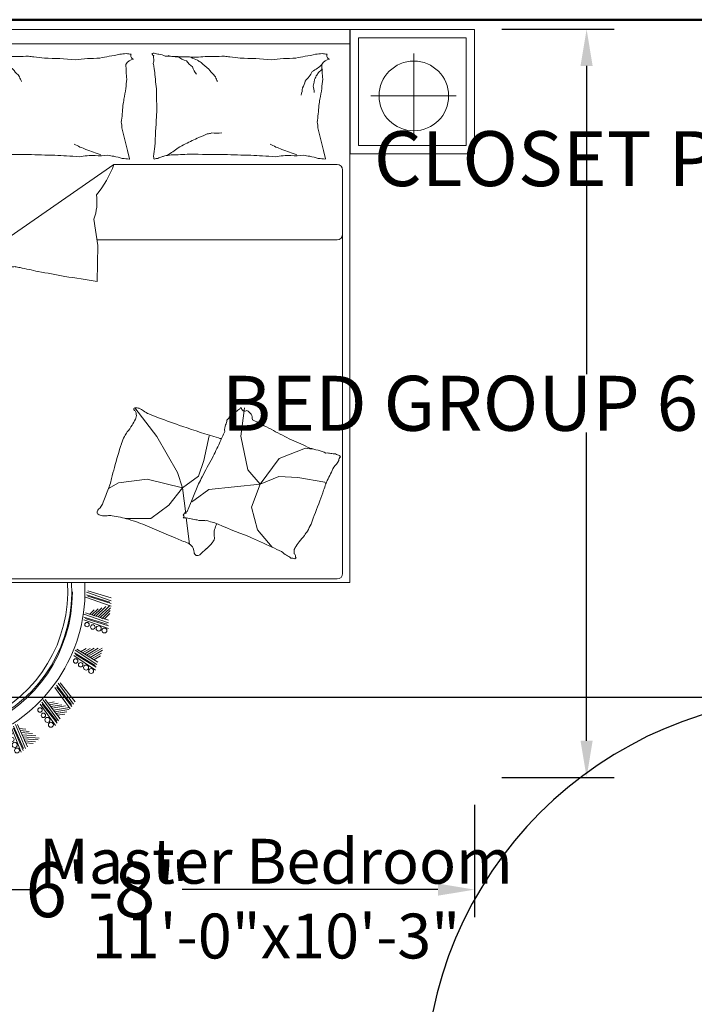
# Model space of a CAD drawing. Units: inches. Extents: x -59 to 502, y -260 to 136.
# Tile 5 of 8: x 77 to 151, y -53 to 55. Entities that reach past the tile are written whole.
import ezdxf

# ---------------------------------------------------------------- set-up
doc = ezdxf.new("R2010")
doc.units = ezdxf.units.IN
doc.header["$MEASUREMENT"] = 0
for name, color, linetype, lineweight in [('A-ANNO-DIMS', 2, 'Continuous', 18), ('A-AREA-IDEN', 7, 'Continuous', 25), ('Beds', 122, 'Continuous', 18), ('Doors', 18, 'Continuous', 25), ('Outer Wall', 10, 'Continuous', 50)]:
    doc.layers.add(name, color=color, linetype=linetype, lineweight=lineweight)
doc.styles.add('DIM_FONT', font='SIMPLEX.shx', dxfattribs={"width": 0.8})
doc.styles.get("Standard").update_dxf_attribs({"font": 'arial.ttf'})
doc.dimstyles.get("Standard").update_dxf_attribs({"dimtxt": 6, "dimasz": 4, "dimexe": 3, "dimexo": 3, "dimgap": 0.09, "dimtad": 0, "dimtih": 1, "dimtoh": 1, "dimdec": 1, "dimzin": 0, "dimdsep": 46, "dimlunit": 3, "dimtxsty": 'Standard', "dimcen": 0.09, "dimadec": 0, "dimazin": 0, "dimtfac": 1, "dimtdec": 1, "dimtofl": 0, "dimtmove": 0, "dimatfit": 3, "dimfxl": 1, "dimtolj": 1, "dimtzin": 0, "dimarcsym": 0})

# ---------------------------------------------------------------- blocks, each defined once
blk = doc.blocks.new('*U11')
for p, q in [((-40, 0), (-40, 6)), ((0, 0), (0, 6))]:
    blk.add_line(p, q)
blk.add_lwpolyline([(0, 0), (0, -40), (-1.75, -40), (-1.75, 0)], close=True)
blk.add_arc((0, 0), 40, 180, 270)
blk = doc.blocks.new('A$C187B6359')
for p, q in [((0.2493, 2.7052), (0.2493, 2.2552)), ((0.6993, 2.7052), (0.2493, 2.7052)), ((0.2793, 2.6752), (0.2793, 2.2852)), ((0.6693, 2.6752), (0.2793, 2.6752)), ((0.6693, 2.2852), (0.6693, 2.6752)), ((0.6993, 2.2552), (0.6993, 2.7052)), ((0.6999, 2.7053), (0.6999, 0.7053)), ((2.1999, 2.7053), (0.6999, 2.7053)), ((2.1999, 0.7053), (2.1999, 2.7053)), ((2.2013, 2.7052), (2.2013, 2.2552)), ((2.6513, 2.7052), (2.2013, 2.7052)), ((2.2313, 2.6752), (2.2313, 2.2852)), ((2.6213, 2.6752), (2.2313, 2.6752)), ((2.6213, 2.2852), (2.6213, 2.6752)), ((2.6513, 2.2552), (2.6513, 2.7052)), ((2.1999, 2.653), (0.6999, 2.653)), ((0.4797, 2.6178), (0.4797, 2.3115)), ((2.4317, 2.6178), (2.4317, 2.3115)), ((0.3236, 2.4648), (0.6327, 2.4648)), ((2.2756, 2.4648), (2.5847, 2.4648)), ((1.3953, 2.267), (1.3747, 2.3496)), ((2.1046, 2.267), (2.0839, 2.3496)), ((0.2793, 2.2852), (0.6693, 2.2852)), ((0.6727, 2.3088), (0.6721, 2.3088)), ((2.2313, 2.2852), (2.6213, 2.2852)), ((0.2493, 2.2552), (0.6993, 2.2552)), ((1.4029, 2.237), (1.3953, 2.267)), ((2.1121, 2.237), (2.1046, 2.267)), ((2.2013, 2.2552), (2.6513, 2.2552)), ((1.3464, 2.2168), (0.7284, 1.7894)), ((1.3464, 2.2168), (2.1541, 2.2168)), ((2.1741, 2.1968), (2.1741, 0.7375)), ((1.2876, 1.9238), (1.2739, 2.0192)), ((2.1541, 1.9442), (1.2846, 1.9442)), ((1.2858, 1.7936), (1.2876, 1.9238)), ((0.7284, 0.7375), (0.7284, 1.7894)), ((0.5264, 1.3215), (0.5217, 1.2334)), ((0.5361, 1.3238), (0.5277, 1.2297)), ((0.5421, 1.3201), (0.5374, 1.232)), ((0.5458, 1.3261), (0.5411, 1.238)), ((0.5555, 1.3284), (0.5471, 1.2343)), ((0.5629, 1.3285), (0.5533, 1.2408)), ((0.6047, 1.292), (0.5545, 1.3229)), ((0.5727, 1.3302), (0.5591, 1.2368)), ((0.6051, 1.3), (0.5613, 1.327)), ((0.5785, 1.3262), (0.5689, 1.2385)), ((0.6077, 1.3067), (0.5719, 1.3288)), ((0.5825, 1.332), (0.5729, 1.2443)), ((0.5923, 1.3337), (0.5787, 1.2403)), ((0.6059, 1.3161), (0.5826, 1.3304)), ((0.6394, 1.2947), (0.5911, 1.3283)), ((0.6403, 1.3027), (0.5981, 1.332)), ((0.6068, 1.3321), (0.6021, 1.244)), ((0.6165, 1.3344), (0.6081, 1.2403)), ((0.6432, 1.3092), (0.6087, 1.3332)), ((0.6225, 1.3307), (0.6178, 1.2426)), ((0.642, 1.3186), (0.6195, 1.3342)), ((0.6262, 1.3367), (0.6215, 1.2486)), ((0.6358, 1.339), (0.6275, 1.2449)), ((0.6437, 1.3345), (0.6342, 1.2469)), ((0.6535, 1.3363), (0.6399, 1.2428)), ((0.6593, 1.3323), (0.6497, 1.2446)), ((0.6633, 1.3381), (0.6538, 1.2504)), ((0.6731, 1.3398), (0.6595, 1.2463)), ((1.4224, 1.3369), (1.5015, 1.233)), ((1.8189, 1.3371), (1.8052, 1.2339)), ((0.3946, 1.283), (0.4199, 1.192)), ((0.4604, 1.2704), (0.4117, 1.2871)), ((0.4614, 1.2774), (0.4216, 1.2911)), ((0.4577, 1.2862), (0.4318, 1.2951)), ((0.455, 1.302), (0.4698, 1.215)), ((0.4639, 1.3064), (0.4764, 1.2128)), ((0.4706, 1.3041), (0.4854, 1.2171)), ((0.4729, 1.3107), (0.4877, 1.2238)), ((0.4818, 1.3151), (0.4943, 1.2215)), ((0.6042, 1.284), (0.5618, 1.3102)), ((0.6049, 1.2753), (0.569, 1.2975)), ((0.6034, 1.268), (0.5762, 1.2848)), ((0.6385, 1.2867), (0.5976, 1.3152)), ((0.6387, 1.278), (0.6041, 1.3021)), ((0.6368, 1.2708), (0.6105, 1.289)), ((0.3378, 1.2518), (0.3728, 1.164)), ((0.3796, 1.2429), (0.3383, 1.2509)), ((0.3747, 1.251), (0.3478, 1.2562)), ((0.3698, 1.2663), (0.3965, 1.1822)), ((0.3781, 1.2719), (0.4034, 1.1809)), ((0.385, 1.2705), (0.4116, 1.1864)), ((0.3863, 1.2774), (0.413, 1.1934)), ((0.4617, 1.2625), (0.406, 1.2816)), ((0.4631, 1.2546), (0.4159, 1.2708)), ((0.4656, 1.2462), (0.4257, 1.2599)), ((0.4657, 1.2388), (0.4355, 1.2491)), ((0.6035, 1.2597), (0.5834, 1.2721)), ((0.6364, 1.2624), (0.617, 1.2759)), ((0.6999, 1.25), (0.641, 1.25)), ((0.3272, 1.2103), (0.2853, 1.2138)), ((0.3214, 1.2178), (0.2942, 1.2201)), ((0.315, 1.2325), (0.3505, 1.1518)), ((0.3226, 1.2389), (0.3575, 1.1512)), ((0.3819, 1.2281), (0.3242, 1.2393)), ((0.3795, 1.2357), (0.3291, 1.2455)), ((0.3296, 1.2383), (0.3651, 1.1576)), ((0.3302, 1.2453), (0.3657, 1.1646)), ((0.3844, 1.2204), (0.3354, 1.23)), ((0.388, 1.2125), (0.3466, 1.2206)), ((0.3892, 1.2052), (0.3578, 1.2113)), ((0.4677, 1.2306), (0.4454, 1.2383)), ((1.5015, 1.233), (1.5767, 1.1026)), ((1.6715, 1.1461), (1.6913, 1.235)), ((1.8052, 1.2339), (1.831, 1.1119)), ((0.2407, 1.1781), (0.2871, 1.1031)), ((0.2474, 1.1856), (0.2941, 1.1035)), ((0.248, 1.1868), (0.2836, 1.1061)), ((0.254, 1.193), (0.3004, 1.1179)), ((0.2544, 1.1859), (0.3008, 1.1109)), ((0.2556, 1.1933), (0.2906, 1.1055)), ((0.2607, 1.2004), (0.3074, 1.1183)), ((0.2626, 1.1927), (0.2982, 1.1119)), ((0.2632, 1.1997), (0.2988, 1.1189)), ((0.2708, 1.2061), (0.3058, 1.1184)), ((0.3311, 1.1958), (0.2725, 1.2008)), ((0.3279, 1.2031), (0.2767, 1.2075)), ((0.3344, 1.1885), (0.2846, 1.1927)), ((0.3389, 1.181), (0.2968, 1.1846)), ((0.3408, 1.1738), (0.309, 1.1765)), ((0.3923, 1.1974), (0.3691, 1.2019)), ((1.9445, 1.1532), (2.0391, 1.191)), ((2.0391, 1.191), (2.0632, 1.1875)), ((0.2007, 1.1459), (0.2474, 1.0638)), ((0.2618, 1.144), (0.203, 1.1409)), ((0.2576, 1.1509), (0.2063, 1.1481)), ((0.2559, 1.1578), (0.2139, 1.1555)), ((0.2492, 1.1645), (0.2218, 1.163)), ((0.3447, 1.1664), (0.3212, 1.1684)), ((1.6518, 1.0888), (1.6715, 1.1461)), ((1.8757, 1.0603), (1.9445, 1.1532)), ((0.1651, 1.1077), (0.2244, 1.0425)), ((0.1678, 1.1099), (0.2241, 1.042)), ((0.1703, 1.1162), (0.2313, 1.0441)), ((0.1733, 1.1182), (0.231, 1.0434)), ((0.1789, 1.1264), (0.2352, 1.0585)), ((0.1802, 1.1195), (0.2366, 1.0516)), ((0.1807, 1.1237), (0.2271, 1.0486)), ((0.1845, 1.1347), (0.2421, 1.0599)), ((0.1874, 1.1311), (0.2341, 1.049)), ((0.194, 1.1385), (0.2404, 1.0634)), ((0.1944, 1.1315), (0.2408, 1.0564)), ((0.266, 1.1372), (0.2162, 1.1345)), ((0.2715, 1.1305), (0.2294, 1.1282)), ((0.2744, 1.1236), (0.2425, 1.1218)), ((0.2793, 1.1168), (0.2557, 1.1155)), ((1.831, 1.1119), (1.8757, 1.0603)), ((0.1734, 1.0735), (0.1325, 1.0636)), ((0.1934, 1.0791), (0.1356, 1.0678)), ((0.1882, 1.0852), (0.1378, 1.0754)), ((0.1655, 1.0789), (0.1389, 1.0724)), ((0.1856, 1.0919), (0.1444, 1.0838)), ((0.1985, 1.0729), (0.1495, 1.0633)), ((0.178, 1.0976), (0.1512, 1.0923)), ((0.1547, 1.0907), (0.2141, 1.0255)), ((0.1599, 1.0992), (0.2209, 1.0271)), ((0.1667, 1.1009), (0.2261, 1.0356)), ((1.466, 1.0789), (1.3632, 1.0651)), ((1.5944, 1.0473), (1.466, 1.0789)), ((1.5767, 1.1026), (1.5944, 1.0473)), ((1.5944, 1.0473), (1.6518, 1.0888)), ((1.8757, 1.0603), (1.9428, 1.0878)), ((1.9428, 1.0878), (2.0116, 1.0844)), ((2.0116, 1.0844), (2.1096, 1.0672)), ((0.1109, 1.0347), (0.1719, 0.9626)), ((0.1133, 1.0342), (0.1792, 0.9755)), ((0.1161, 1.0432), (0.1754, 0.9779)), ((0.1176, 1.0432), (0.1858, 0.9779)), ((0.1178, 1.0363), (0.1771, 0.9711)), ((0.1213, 1.0517), (0.1823, 0.9796)), ((0.1218, 1.0522), (0.1877, 0.9935)), ((0.1242, 1.0456), (0.1901, 0.9869)), ((0.1817, 1.0611), (0.1245, 1.0471)), ((0.1261, 1.0612), (0.1943, 0.9959)), ((0.1763, 1.067), (0.1264, 1.0548)), ((0.1871, 1.0551), (0.1386, 1.0433)), ((0.1937, 1.0495), (0.1527, 1.0395)), ((0.2049, 1.067), (0.1634, 1.0589)), ((0.1979, 1.0433), (0.1668, 1.0357)), ((0.2087, 1.0605), (0.1774, 1.0544)), ((0.2039, 1.0375), (0.181, 1.0319)), ((0.2145, 1.0545), (0.1913, 1.05)), ((1.3632, 1.0651), (1.3272, 1.045)), ((1.545, 0.9841), (1.5944, 1.0473)), ((1.5944, 1.0473), (1.6062, 0.9532)), ((1.6527, 1.0611), (1.6296, 1.0048)), ((1.6899, 1.0414), (1.64, 1.0053)), ((1.8757, 1.0603), (1.6899, 1.0414)), ((1.8447, 0.9778), (1.8757, 1.0603)), ((2.1096, 1.0672), (2.1129, 1.0608)), ((0.0871, 0.9983), (0.1598, 0.938)), ((0.1433, 1.0075), (0.0879, 0.9877)), ((0.0879, 1.0018), (0.1627, 0.9441)), ((0.088, 0.9985), (0.1592, 0.9463)), ((0.1373, 1.0129), (0.0889, 0.9955)), ((0.0907, 1.0076), (0.1605, 0.9537)), ((0.0914, 1.0078), (0.1656, 0.9493)), ((0.0935, 1.0012), (0.1634, 0.9473)), ((0.1337, 1.0191), (0.0941, 1.0049)), ((0.0943, 1.0169), (0.167, 0.9566)), ((0.1253, 1.0235), (0.0995, 1.0143)), ((0.1493, 1.0022), (0.1023, 0.9854)), ((0.1057, 1.0262), (0.1651, 0.9609)), ((0.1564, 0.9973), (0.1167, 0.9831)), ((1.6296, 1.0048), (1.6119, 0.9614)), ((1.64, 1.0053), (1.628, 0.9967)), ((0.1152, 0.9646), (0.0614, 0.9409)), ((0.1089, 0.9695), (0.0618, 0.9488)), ((0.103, 0.9666), (0.0649, 0.9487)), ((0.1049, 0.9754), (0.0664, 0.9585)), ((0.0911, 0.9643), (0.0665, 0.9524)), ((0.0942, 0.9703), (0.0694, 0.9586)), ((0.0962, 0.9793), (0.0711, 0.9683)), ((0.0714, 0.9648), (0.1373, 0.9062)), ((0.0756, 0.9738), (0.1439, 0.9085)), ((0.0781, 0.9736), (0.1498, 0.9222)), ((0.0799, 0.9828), (0.1458, 0.9242)), ((0.0813, 0.9797), (0.1524, 0.9276)), ((0.0814, 0.983), (0.1561, 0.9253)), ((0.0823, 0.9762), (0.1482, 0.9175)), ((0.0835, 0.9891), (0.1533, 0.9352)), ((0.0842, 0.9918), (0.1524, 0.9266)), ((0.0847, 0.9924), (0.1563, 0.941)), ((0.0847, 0.9891), (0.1588, 0.9306)), ((0.0877, 0.9861), (0.1594, 0.9347)), ((0.091, 0.9921), (0.1622, 0.94)), ((0.1612, 0.9915), (0.1312, 0.9808)), ((0.1678, 0.9864), (0.1456, 0.9784)), ((1.4798, 0.9367), (1.545, 0.9841)), ((1.8654, 0.8953), (1.8447, 0.9778)), ((0.0535, 0.9284), (0.1283, 0.8707)), ((0.054, 0.9291), (0.1307, 0.8855)), ((0.0563, 0.9387), (0.1367, 0.8892)), ((0.0563, 0.9348), (0.1304, 0.8763)), ((0.1107, 0.9503), (0.0577, 0.9247)), ((0.1042, 0.9549), (0.0579, 0.9326)), ((0.1136, 0.956), (0.0603, 0.931)), ((0.1071, 0.9608), (0.0606, 0.9389)), ((0.0999, 0.9607), (0.0621, 0.9424)), ((0.1172, 0.9456), (0.0723, 0.9239)), ((0.1201, 0.9513), (0.0749, 0.9301)), ((0.1216, 0.9597), (0.0759, 0.9396)), ((0.1249, 0.9415), (0.0869, 0.9231)), ((0.1277, 0.9471), (0.0895, 0.9292)), ((0.1291, 0.9553), (0.0905, 0.9383)), ((0.1302, 0.9362), (0.1015, 0.9224)), ((0.133, 0.9418), (0.1041, 0.9282)), ((0.1343, 0.9499), (0.105, 0.937)), ((0.1373, 0.9318), (0.116, 0.9216)), ((0.1401, 0.9374), (0.1187, 0.9273)), ((0.1412, 0.9452), (0.1196, 0.9357)), ((1.3869, 0.9367), (1.4798, 0.9367)), ((1.6081, 0.9385), (1.6199, 0.8439)), ((0.0773, 0.8938), (0.0336, 0.8667)), ((0.0725, 0.8991), (0.0368, 0.877)), ((0.0634, 0.9017), (0.0401, 0.8873)), ((0.0437, 0.9002), (0.1154, 0.8488)), ((0.0461, 0.9067), (0.1173, 0.8546)), ((0.047, 0.9096), (0.1217, 0.8519)), ((0.0494, 0.9097), (0.1261, 0.8661)), ((0.0495, 0.9161), (0.1236, 0.8576)), ((0.0503, 0.919), (0.122, 0.8676)), ((0.0517, 0.9194), (0.1321, 0.8698)), ((0.0529, 0.9254), (0.124, 0.8733)), ((0.0533, 0.9127), (0.125, 0.8613)), ((0.0559, 0.9191), (0.127, 0.8669)), ((0.0577, 0.9231), (0.1344, 0.8795)), ((1.919, 0.8327), (1.8654, 0.8953)), ((0.0298, 0.8621), (0.1102, 0.8126)), ((0.0301, 0.8628), (0.111, 0.8276)), ((0.0314, 0.8727), (0.1166, 0.8319)), ((0.0843, 0.8899), (0.0343, 0.8589)), ((0.0345, 0.8573), (0.1153, 0.822)), ((0.0913, 0.8859), (0.0489, 0.8596)), ((0.0993, 0.8826), (0.0635, 0.8604)), ((0.1052, 0.878), (0.0781, 0.8612)), ((0.1127, 0.8744), (0.0927, 0.8619)), ((0.0571, 0.8302), (0.0165, 0.7987)), ((0.0165, 0.8199), (0.0992, 0.7892)), ((0.0171, 0.8298), (0.1045, 0.7938)), ((0.0644, 0.827), (0.0179, 0.7909)), ((0.0517, 0.835), (0.0185, 0.8092)), ((0.0424, 0.8367), (0.0208, 0.8199)), ((0.023, 0.8331), (0.0997, 0.7895)), ((0.0252, 0.8428), (0.1056, 0.7932)), ((0.0275, 0.8525), (0.1042, 0.8089)), ((0.0277, 0.8431), (0.1085, 0.8078)), ((0.0289, 0.8529), (0.1141, 0.8121)), ((0.0312, 0.8465), (0.1079, 0.8029)), ((0.0718, 0.8238), (0.0324, 0.7932)), ((0.0801, 0.8214), (0.0468, 0.7955)), ((0.0452, 0.7888), (0.0064, 0.7551)), ((0.0396, 0.7933), (0.0079, 0.7657)), ((0.0527, 0.7861), (0.0083, 0.7474)), ((0.0301, 0.7944), (0.0095, 0.7765)), ((0.0119, 0.7839), (0.0927, 0.7486)), ((0.0131, 0.7937), (0.0983, 0.7529)), ((0.0151, 0.8), (0.0978, 0.7693)), ((0.0158, 0.8099), (0.1031, 0.774)), ((0.0211, 0.8145), (0.1038, 0.7839)), ((0.0865, 0.8174), (0.0612, 0.7978)), ((0.0943, 0.8146), (0.0757, 0.8001)), ((0.0094, 0.7641), (0.0902, 0.7289)), ((0.0106, 0.774), (0.0958, 0.7332)), ((0.0162, 0.7783), (0.0971, 0.743)), ((0.0602, 0.7833), (0.0226, 0.7505)), ((0.0687, 0.7813), (0.0369, 0.7536)), ((0.0752, 0.7777), (0.0512, 0.7567)), ((0.0832, 0.7753), (0.0654, 0.7598)), ((2.1541, 0.7175), (0.7484, 0.7175)), ((0.6999, 0.7053), (2.1999, 0.7053)), ((0, 0.6734), (0.0935, 0.6598)), ((0.0018, 0.6636), (0.0894, 0.654)), ((0.0035, 0.6538), (0.097, 0.6402)), ((0.0053, 0.644), (0.093, 0.6344)), ((0.0212, 0.6423), (0.0056, 0.6198)), ((0.0306, 0.6435), (0.0066, 0.609)), ((0.0075, 0.6596), (0.0952, 0.65)), ((1.336, 0.619), (1.243, 0.6516)), ((1.3313, 0.6341), (1.2471, 0.6602)), ((1.3363, 0.639), (1.2472, 0.6702)), ((1.3362, 0.629), (1.252, 0.6552)), ((1.3365, 0.6489), (1.2523, 0.6751)), ((0.0372, 0.6405), (0.0078, 0.5983)), ((0.0451, 0.6396), (0.0115, 0.5913)), ((0.0531, 0.6388), (0.0246, 0.5978)), ((0.0618, 0.639), (0.0377, 0.6043)), ((0.069, 0.637), (0.0508, 0.6108)), ((0.0774, 0.6367), (0.0639, 0.6173)), ((1.2576, 0.5894), (1.2746, 0.6058)), ((1.2657, 0.5875), (1.2887, 0.6097)), ((1.2725, 0.5842), (1.3028, 0.6136)), ((1.281, 0.5827), (1.3169, 0.6174)), ((1.2887, 0.5803), (1.331, 0.6213)), ((1.2964, 0.5779), (1.3333, 0.6137)), ((0.0061, 0.5926), (0.0995, 0.579)), ((0.0078, 0.5828), (0.0955, 0.5732)), ((0.0096, 0.573), (0.1031, 0.5594)), ((0.0136, 0.5788), (0.1013, 0.5692)), ((1.3218, 0.5536), (1.2375, 0.5798)), ((1.3268, 0.5585), (1.2377, 0.5897)), ((1.3267, 0.5485), (1.2424, 0.5747)), ((1.327, 0.5684), (1.2428, 0.5946)), ((1.3022, 0.5738), (1.3324, 0.6031)), ((1.3117, 0.5732), (1.3313, 0.5922)), ((0.0113, 0.5632), (0.099, 0.5536)), ((1.3265, 0.5386), (1.2374, 0.5698)), ((0.0247, 0.4821), (0.1183, 0.4946)), ((0.0291, 0.4731), (0.116, 0.4879)), ((0.0334, 0.4642), (0.1271, 0.4767)), ((0.0357, 0.4708), (0.1227, 0.4857)), ((0.0378, 0.4552), (0.1248, 0.47)), ((0.0853, 0.4633), (0.0691, 0.4161)), ((0.0936, 0.4659), (0.0799, 0.426)), ((0.1011, 0.466), (0.0907, 0.4358)), ((0.1092, 0.468), (0.1015, 0.4456)), ((1.2875, 0.4172), (1.2122, 0.4631)), ((1.2253, 0.4544), (1.2458, 0.4663)), ((1.2327, 0.4506), (1.2604, 0.4666)), ((1.2385, 0.4458), (1.275, 0.4669)), ((1.2464, 0.4422), (1.2896, 0.4672)), ((1.2533, 0.4381), (1.3042, 0.4675)), ((0.0536, 0.4579), (0.0448, 0.4321)), ((0.0624, 0.4617), (0.0487, 0.4219)), ((0.0694, 0.4606), (0.0528, 0.412)), ((0.0773, 0.462), (0.0582, 0.4063)), ((1.2798, 0.3883), (1.2009, 0.4403)), ((1.2788, 0.4041), (1.2035, 0.45)), ((1.2849, 0.4076), (1.2061, 0.4596)), ((1.2824, 0.398), (1.207, 0.4439)), ((1.2601, 0.4339), (1.3046, 0.4596)), ((1.2647, 0.4284), (1.3012, 0.4495)), ((1.2738, 0.4255), (1.2975, 0.4392)), ((0.0881, 0.3381), (0.1758, 0.373)), ((0.0945, 0.3304), (0.1752, 0.366)), ((0.1009, 0.3228), (0.1886, 0.3578)), ((0.1015, 0.3299), (0.1822, 0.3654)), ((0.1073, 0.3152), (0.188, 0.3508)), ((0.122, 0.3217), (0.1197, 0.2944)), ((0.1296, 0.3275), (0.126, 0.2856)), ((0.1367, 0.3282), (0.1323, 0.2769)), ((0.144, 0.3314), (0.139, 0.2727)), ((0.1514, 0.3346), (0.1471, 0.2849)), ((0.1588, 0.3391), (0.1552, 0.2971)), ((0.166, 0.3411), (0.1633, 0.3093)), ((0.1734, 0.345), (0.1714, 0.3214)), ((1.1882, 0.2484), (1.1328, 0.3249)), ((1.1929, 0.2635), (1.1386, 0.333)), ((1.194, 0.2565), (1.1397, 0.3261)), ((1.1998, 0.2646), (1.1444, 0.3411)), ((1.2056, 0.2727), (1.1513, 0.3422)), ((0.1337, 0.2711), (0.2215, 0.3061)), ((0.1401, 0.2635), (0.2209, 0.299)), ((0.1466, 0.2559), (0.2343, 0.2908)), ((0.1472, 0.2629), (0.2279, 0.2985)), ((0.153, 0.2483), (0.2337, 0.2838)), ((1.1345, 0.1877), (1.0791, 0.2642)), ((1.1392, 0.2028), (1.0849, 0.2723)), ((1.1403, 0.1958), (1.086, 0.2653)), ((1.1461, 0.2039), (1.0907, 0.2804)), ((1.1519, 0.212), (1.0976, 0.2815)), ((1.1069, 0.2688), (1.1302, 0.2726)), ((1.1124, 0.2626), (1.144, 0.2678)), ((1.1161, 0.256), (1.1577, 0.2629)), ((1.1223, 0.2499), (1.1715, 0.2581)), ((1.1272, 0.2436), (1.1853, 0.2532)), ((1.1322, 0.2373), (1.1829, 0.2457)), ((1.1346, 0.2306), (1.1761, 0.2374)), ((1.142, 0.2247), (1.169, 0.2291)), ((0.2468, 0.148), (0.3166, 0.2116)), ((0.2555, 0.1431), (0.3185, 0.2048)), ((0.2623, 0.145), (0.3253, 0.2068)), ((0.2642, 0.1382), (0.334, 0.2019)), ((0.2729, 0.1334), (0.3359, 0.1951)), ((0.3187, 0.1783), (0.3274, 0.1475)), ((0.3243, 0.1845), (0.3307, 0.1618)), ((1.0105, 0.0909), (0.9754, 0.1786)), ((1.0187, 0.1044), (0.9829, 0.185)), ((1.0257, 0.1038), (0.9905, 0.1915)), ((1.0333, 0.1102), (0.9976, 0.1909)), ((0.2843, 0.1446), (0.2918, 0.1183)), ((0.2894, 0.1527), (0.3008, 0.1122)), ((0.2958, 0.1558), (0.3098, 0.1064)), ((0.3015, 0.1614), (0.3176, 0.1048)), ((0.3073, 0.1671), (0.3208, 0.1191)), ((0.3126, 0.1739), (0.3241, 0.1333)), ((0.3809, 0.0657), (0.4331, 0.1445)), ((1.0181, 0.0974), (0.9824, 0.178)), ((1.0034, 0.1763), (1.027, 0.1743)), ((1.0073, 0.1689), (1.0391, 0.1663)), ((1.0093, 0.1617), (1.0513, 0.1582)), ((1.0138, 0.1542), (1.0635, 0.1501)), ((1.017, 0.1469), (1.0757, 0.1421)), ((0.3906, 0.0631), (0.4366, 0.1384)), ((0.3967, 0.0666), (0.4427, 0.1419)), ((0.4002, 0.0605), (0.4524, 0.1393)), ((0.4098, 0.0579), (0.4559, 0.1332)), ((0.4385, 0.1069), (0.4595, 0.0703)), ((0.4433, 0.1127), (0.4592, 0.085)), ((0.4472, 0.12), (0.4589, 0.0996)), ((0.4566, 0.0367), (0.5088, 0.1155)), ((0.4662, 0.0341), (0.5123, 0.1094)), ((0.4723, 0.0377), (0.5184, 0.1129)), ((0.4759, 0.0315), (0.528, 0.1103)), ((0.7956, 0.0156), (0.7936, 0.11)), ((0.805, 0.0189), (0.7999, 0.107)), ((0.8555, 0.0282), (0.8535, 0.1226)), ((0.8649, 0.0315), (0.8599, 0.1196)), ((0.8679, 0.0379), (0.8629, 0.1259)), ((0.8743, 0.0349), (0.8723, 0.1293)), ((0.8837, 0.0382), (0.8787, 0.1263)), ((1.0203, 0.1396), (1.0715, 0.1353)), ((1.021, 0.1325), (1.0629, 0.129)), ((1.0268, 0.1249), (1.0541, 0.1227)), ((0.4182, 0.0716), (0.4318, 0.0479)), ((0.4211, 0.0807), (0.442, 0.0442)), ((0.4265, 0.0853), (0.4522, 0.0407)), ((0.4307, 0.0921), (0.4601, 0.0411)), ((0.4349, 0.099), (0.4598, 0.0557)), ((0.4855, 0.029), (0.5315, 0.1042)), ((0.6197, 0), (0.6408, 0.0921)), ((0.6296, 0.001), (0.6463, 0.0876)), ((0.6341, 0.0064), (0.6507, 0.093)), ((0.6396, 0.0019), (0.6606, 0.094)), ((0.6495, 0.0029), (0.6661, 0.0895)), ((0.6626, 0.0742), (0.6808, 0.0592)), ((0.7768, 0.0089), (0.7748, 0.1033)), ((0.7862, 0.0122), (0.7812, 0.1003)), ((0.7892, 0.0186), (0.7842, 0.1066)), ((0.8003, 0.0912), (0.8216, 0.0811)), ((0.8006, 0.0755), (0.8387, 0.0574)), ((0.8013, 0.083), (0.8302, 0.0693)), ((0.657, 0.0423), (0.7025, 0.0049)), ((0.6585, 0.0501), (0.697, 0.0184)), ((0.659, 0.0588), (0.6916, 0.032)), ((0.6615, 0.0659), (0.6862, 0.0456)), ((0.8013, 0.044), (0.8393, 0.026)), ((0.8022, 0.0669), (0.8473, 0.0456)), ((0.8027, 0.0589), (0.8559, 0.0337)), ((0.8031, 0.0509), (0.8496, 0.0289)), ((0.652, 0.0281), (0.6845, 0.0014)), ((0.6525, 0.0186), (0.6736, 0.0013)), ((0.6555, 0.0344), (0.6952, 0.0017)), ((0.804, 0.0349), (0.8288, 0.0232))]:
    blk.add_line(p, q)
for centre, radius in [((0.4797, 2.4648), 0.126), ((2.4317, 2.4648), 0.126), ((0.6466, 1.3265), 0.00895), ((0.6832, 1.3267), 0.00895), ((0.409, 1.2751), 0.00895), ((0.495, 1.3053), 0.00895), ((0.4979, 1.2836), 0.00929), ((0.6447, 1.3047), 0.00929), ((0.6447, 1.2827), 0.00801), ((0.68, 1.3051), 0.00929), ((0.6788, 1.2831), 0.00801), ((0.353, 1.2454), 0.00895), ((0.4149, 1.254), 0.00929), ((0.5028, 1.2622), 0.00801), ((0.5045, 1.2395), 0.00801), ((0.6414, 1.2602), 0.00801), ((0.6743, 1.2609), 0.00801), ((0.3611, 1.2251), 0.00929), ((0.3711, 1.2055), 0.00801), ((0.4227, 1.2335), 0.00801), ((0.4275, 1.2112), 0.00801), ((0.2766, 1.1962), 0.00895), ((0.2875, 1.1772), 0.00929), ((0.3783, 1.184), 0.00801), ((0.2008, 1.1328), 0.00895), ((0.3, 1.1592), 0.00801), ((0.3101, 1.1388), 0.00801), ((0.1867, 1.1151), 0.00895), ((0.2008, 1.0984), 0.00929), ((0.2142, 1.1155), 0.00929), ((0.2291, 1.0994), 0.00801), ((0.1426, 1.0618), 0.00895), ((0.2165, 1.083), 0.00801), ((0.2301, 1.0648), 0.00801), ((0.2419, 1.0806), 0.00801), ((0.1584, 1.0467), 0.00929), ((0.1756, 1.033), 0.00801), ((0.1043, 1.0041), 0.00895), ((0.1078, 1.01), 0.00895), ((0.1107, 1.0186), 0.00895), ((0.1216, 0.9908), 0.00929), ((0.1249, 0.9964), 0.00929), ((0.1276, 1.0047), 0.00929), ((0.1457, 0.9922), 0.00801), ((0.1911, 1.0163), 0.00801), ((0.1401, 0.979), 0.00801), ((0.1434, 0.9844), 0.00801), ((0.1573, 0.964), 0.00801), ((0.1604, 0.9693), 0.00801), ((0.1623, 0.9767), 0.00801), ((0.0722, 0.9428), 0.00895), ((0.0909, 0.9313), 0.00929), ((0.1106, 0.9215), 0.00801), ((0.1292, 0.9085), 0.00801), ((0.0469, 0.8784), 0.00895), ((0.0666, 0.8689), 0.00929), ((0.0872, 0.8613), 0.00801), ((0.1071, 0.8503), 0.00801), ((0.0323, 0.8363), 0.00895), ((0.0525, 0.828), 0.00929), ((0.0735, 0.8215), 0.00801), ((0.094, 0.8117), 0.00801), ((0.0131, 0.6834), 0.00895), ((0.0347, 0.6803), 0.00929), ((0.0567, 0.6791), 0.00801), ((0.079, 0.6745), 0.00801), ((1.2488, 0.5526), 0.00801), ((1.2698, 0.5438), 0.00801), ((1.2911, 0.5385), 0.00929), ((1.3118, 0.5312), 0.00895), ((0.0345, 0.4953), 0.00895), ((0.0562, 0.4982), 0.00929), ((0.0777, 0.5031), 0.00801), ((0.1003, 0.5048), 0.00801), ((1.2078, 0.4208), 0.00801), ((1.226, 0.4072), 0.00801), ((1.2454, 0.3969), 0.00929), ((1.2637, 0.3848), 0.00895), ((0.0944, 0.3533), 0.00895), ((0.1147, 0.3614), 0.00929), ((0.1343, 0.3714), 0.00801), ((0.1559, 0.3785), 0.00801), ((1.0786, 0.2435), 0.00801), ((0.296, 0.2097), 0.00801), ((1.0909, 0.2244), 0.00801), ((1.1054, 0.2078), 0.00929), ((0.2635, 0.1792), 0.00929), ((0.2784, 0.1954), 0.00801), ((1.1182, 0.1901), 0.00895), ((0.2474, 0.1644), 0.00895), ((0.4136, 0.1376), 0.00801), ((0.9699, 0.1587), 0.00801), ((0.9771, 0.1371), 0.00801), ((0.3895, 0.1001), 0.00929), ((0.4, 0.1194), 0.00801), ((0.9871, 0.1175), 0.00929), ((0.3775, 0.0818), 0.00895), ((0.625, 0.0788), 0.00801), ((0.7618, 0.0638), 0.00801), ((0.7627, 0.0865), 0.00801), ((0.9953, 0.0972), 0.00895), ((0.6157, 0.0352), 0.00929), ((0.6186, 0.057), 0.00801), ((0.7643, 0.042), 0.00929), ((0.6108, 0.0139), 0.00895), ((0.7648, 0.0201), 0.00895)]:
    blk.add_circle(centre, radius)
for centre, radius, start, end in [((0.7725, 2.6193), 0.00342, 291.7883, 340.436), ((0.7743, 2.6138), 0.00232, 340.436, 101.8931), ((0.7738, 2.6432), 0.0251, 274.3025, 291.7883), ((0.7804, 2.6146), 0.00428, 201.9904, 281.8931), ((0.7958, 2.6048), 0.0156, 158.579, 201.9904), ((0.7979, 2.6447), 0.0289, 239.3487, 274.3025), ((0.7951, 2.5622), 0.0539, 59.3487, 84.7408), ((0.7953, 1.7882), 0.8208, 84.7408, 88.0921), ((0.8611, 2.7059), 0.0992, 254.0648, 274.2159), ((0.9268, 2.6871), 0.0992, 233.9136, 254.0648), ((0.8855, 1.1114), 1.4943, 88.0921, 90.5757), ((1.023, 2.8128), 0.234, 242.7604, 249.1397), ((1.0084, 1.7347), 0.8732, 90.5757, 94.8018), ((1.0124, 2.8973), 0.2897, 267.4614, 274.8018), ((1.0636, 2.7586), 0.1524, 259.8101, 267.4614), ((1.0008, 2.08), 0.5293, 79.8101, 83.9133), ((1.0944, 1.552), 1.049, 83.9133, 90), ((1.2953, 1.9183), 0.6827, 90, 97.5469), ((1.361, 2.3678), 0.2422, 97.5469, 105.744), ((1.2845, 2.9094), 0.3048, 278.4372, 285.744), ((1.3672, 2.7772), 0.1611, 270, 278.4372), ((1.4085, 2.7065), 0.0904, 258.7276, 270), ((1.4202, 2.6102), 0.0131, 153.4195, 258.7276), ((1.4817, 2.6193), 0.00342, 291.7883, 340.436), ((1.4835, 2.6138), 0.00232, 340.436, 101.8931), ((1.4831, 2.6432), 0.0251, 274.3025, 291.7883), ((1.4896, 2.6146), 0.00428, 201.9904, 281.8931), ((1.505, 2.6048), 0.0156, 158.579, 201.9904), ((1.5071, 2.6447), 0.0289, 239.3487, 274.3025), ((1.5043, 2.5622), 0.0539, 59.3487, 84.7408), ((1.5045, 1.7882), 0.8208, 84.7408, 88.0921), ((1.5703, 2.7059), 0.0992, 254.0648, 274.2159), ((1.6361, 2.6871), 0.0992, 233.9136, 254.0648), ((1.5948, 1.1114), 1.4943, 88.0921, 90.5757), ((1.7322, 2.8128), 0.234, 242.7604, 249.1397), ((1.7176, 1.7347), 0.8732, 90.5757, 94.8018), ((1.7217, 2.8973), 0.2897, 267.4614, 274.8018), ((1.7729, 2.7586), 0.1524, 259.8101, 267.4614), ((1.71, 2.08), 0.5293, 79.8101, 83.9133), ((1.8036, 1.552), 1.049, 83.9133, 90), ((2.0045, 1.9183), 0.6827, 90, 97.5469), ((2.0703, 2.3678), 0.2422, 97.5469, 105.744), ((1.9937, 2.9094), 0.3048, 278.4372, 285.744), ((2.0764, 2.7772), 0.1611, 270, 278.4372), ((2.1177, 2.7065), 0.0904, 258.7276, 270), ((2.1295, 2.6102), 0.0131, 153.4195, 258.7276), ((0.7489, 2.5943), 0.0328, 338.579, 8.1335), ((0.5389, 2.5307), 0.246, 8.1335, 12.1095), ((0.979, 2.592), 0.1983, 187.6809, 192.1095), ((0.9797, 2.6502), 0.0992, 216.1766, 233.9136), ((1.0154, 2.6015), 0.0992, 198.4397, 216.1766), ((0.9873, 2.6543), 0.0768, 231.6114, 242.7604), ((1.2233, 2.8687), 0.3916, 226.1885, 231.6114), ((1.4203, 2.5633), 0.0342, 94.4002, 153.4195), ((1.8817, 2.5789), 0.4918, 180, 186.2324), ((1.4581, 2.5943), 0.0328, 338.579, 8.1335), ((1.2481, 2.5307), 0.246, 8.1335, 12.1095), ((1.6882, 2.592), 0.1983, 187.6809, 192.1095), ((1.6889, 2.6502), 0.0992, 216.1766, 233.9136), ((1.7246, 2.6015), 0.0992, 198.4397, 216.1766), ((1.6966, 2.6543), 0.0768, 231.6114, 242.7604), ((1.9325, 2.8687), 0.3916, 226.1885, 231.6114), ((2.0003, 2.6777), 0.1399, 297.2036, 314.9024), ((2.1295, 2.5633), 0.0342, 94.4002, 153.4195), ((2.5909, 2.5789), 0.4918, 180, 186.2324), ((1.6965, 2.6041), 0.9131, 183.3687, 187.6809), ((1.155, 2.7035), 0.2252, 219.0349, 226.1885), ((1.0425, 2.5644), 0.0493, 208.3168, 219.0349), ((1.1885, 2.6116), 0.2002, 203.0028, 208.3168), ((2.4058, 2.6041), 0.9131, 183.3687, 187.6809), ((1.8643, 2.7035), 0.2252, 219.0349, 226.1885), ((1.7518, 2.5644), 0.0493, 208.3168, 219.0349), ((1.8977, 2.6116), 0.2002, 203.0028, 208.3168), ((1.9401, 2.6176), 0.1399, 314.9024, 332.6012), ((1.8799, 2.5949), 0.2056, 338.1851, 341.2201), ((1.938, 2.5934), 0.1511, 334.6449, 338.1851), ((2.0389, 2.5721), 0.0526, 318.5571, 334.6449), ((2.0333, 2.622), 0.0899, 306.2641, 318.5571), ((1.5938, 2.4911), 0.204, 170.3156, 180), ((1.8897, 2.5076), 0.1399, 343.485, 354.3689), ((1.9047, 2.5583), 0.1399, 332.6012, 343.485), ((2.0146, 2.5185), 0.0562, 341.2201, 0), ((1.9793, 2.4772), 0.0915, 0, 14.6851), ((2.3031, 2.4911), 0.204, 170.3156, 180), ((1.4701, 2.4627), 0.6787, 178.3669, 183.3687), ((2.252, 2.3048), 0.882, 167.8016, 170.3156), ((2.1793, 2.4627), 0.6787, 178.3669, 183.3687), ((2.9612, 2.3048), 0.882, 167.8016, 170.3156), ((2.1558, 2.35), 1.3652, 176.945, 178.3669), ((0.7204, 2.4609), 0.6588, 351.9949, 357.3351), ((1.0685, 2.4973), 0.3171, 347.8016, 351.9949), ((2.8651, 2.35), 1.3652, 176.945, 178.3669), ((1.4296, 2.4609), 0.6588, 351.9949, 357.3351), ((1.7777, 2.4973), 0.3171, 347.8016, 351.9949), ((14.4012, 1.5554), 13.6356, 176.49514, 176.94504), ((15.1105, 1.5554), 13.6356, 176.49514, 176.94504), ((1.3071, 2.3528), 0.0677, 357.3351, 14.0452), ((2.0163, 2.3528), 0.0677, 357.3351, 14.0452), ((1.4752, 2.7888), 0.5066, 290.6743, 294.3265), ((1.6798, 2.3849), 0.058, 274.0828, 290.6743), ((1.7172, 2.6022), 0.2721, 266.4448, 274.0828), ((1.1013, 2.2263), 0.3212, 170.0016, 176.4951), ((0.9076, 1.6121), 0.7387, 64.6889, 66.5156), ((0.9508, 1.5933), 0.7387, 66.5156, 68.3423), ((1.8106, 2.2263), 0.3212, 170.0016, 176.4951), ((1.4388, 2.5562), 0.3126, 296.4985, 302.135), ((1.0151, 3.5966), 1.4323, 294.3265, 296.4985), ((1.6168, 1.6121), 0.7387, 64.6889, 66.5156), ((1.66, 1.5933), 0.7387, 66.5156, 68.3423), ((0.7623, 2.2404), 0.0193, 350.0016, 16.6978), ((0.8315, 2.1707), 0.0767, 106.2212, 117.2841), ((0.8, 2.2885), 0.0453, 282.869, 297.2841), ((0.8116, 2.3939), 0.1459, 273.574, 282.869), ((0.8383, 3.4157), 1.164, 270.2865, 273.574), ((1.0077, 7.9716), 5.7185, 269.0296, 270.2865), ((1.1894, 5.6119), 3.3622, 267.3904, 269.0296), ((1.2304, 3.4627), 1.2165, 265.3824, 267.3904), ((1.1076, 0.8443), 1.4048, 85.3824, 87.2509), ((1.2668, 2.0191), 0.2301, 87.2509, 101.5586), ((0.9994, 1.5742), 0.7387, 68.3423, 70.572), ((1.0536, 1.5551), 0.7387, 70.572, 72.8018), ((1.2942, 2.3939), 0.1459, 263.5659, 281.5586), ((1.3592, 2.3652), 0.1197, 252.6136, 263.5659), ((1.3079, 2.0197), 0.2297, 72.6136, 80.5159), ((1.4715, 2.2404), 0.0193, 350.0016, 16.6978), ((1.5407, 2.1707), 0.0767, 106.2212, 117.2841), ((1.5092, 2.2885), 0.0453, 282.869, 297.2841), ((1.5209, 2.3939), 0.1459, 273.574, 282.869), ((1.1518, 2.8671), 0.7286, 302.135, 305.8263), ((1.5475, 3.4157), 1.164, 270.2865, 273.574), ((1.7169, 7.9716), 5.7185, 269.0296, 270.2865), ((1.8986, 5.6119), 3.3622, 267.3904, 269.0296), ((1.9396, 3.4627), 1.2165, 265.3824, 267.3904), ((1.8169, 0.8443), 1.4048, 85.3824, 87.2509), ((1.976, 2.0191), 0.2301, 87.2509, 101.5586), ((1.7087, 1.5742), 0.7387, 68.3423, 70.572), ((1.7629, 1.5551), 0.7387, 70.572, 72.8018), ((2.0034, 2.3939), 0.1459, 263.5659, 281.5586), ((2.0684, 2.3652), 0.1197, 252.6136, 263.5659), ((2.0172, 2.0197), 0.2297, 72.6136, 80.5159), ((0.7815, 2.2357), 0.00132, 16.6978, 97.1204), ((0.8072, 2.1521), 0.0875, 97.1204, 106.2212), ((0.9943, 2.346), 0.3751, 320.3555, 339.8512), ((1.3573, 1.9688), 0.2708, 80.5159, 85.9171), ((1.4028, 2.2361), 0.000917, 85.9171, 194.0449), ((1.4907, 2.2357), 0.00132, 16.6978, 97.1204), ((1.5164, 2.1521), 0.0875, 97.1204, 106.2212), ((2.0665, 1.9688), 0.2708, 80.5159, 85.9171), ((2.112, 2.2361), 0.000917, 85.9171, 194.0449), ((2.1541, 2.1968), 0.02, 0, 90), ((1.1048, 2.0812), 0.1801, 339.8512, 8.1356), ((2.1541, 1.9642), 0.02, 270, 0), ((0.0604, 5.8083), 4.0646, 280.7276, 282.9255), ((0.9774, 1.9043), 0.0581, 262.2696, 280.7276), ((1.0326, 2.0362), 0.1942, 256.8096, 262.2696), ((0.4974, -0.6199), 2.5158, 76.8096, 78.3259), ((0.6445, -0.723), 2.588, 78.3259, 80.505), ((0.2245, 3.554), 1.8351, 285.9352, 287.7364), ((0.6365, 2.4469), 0.6574, 282.9255, 285.9352), ((0.6623, -1.9346), 3.7801, 80.505, 82.308), ((1.4245, 1.3321), 0.0063, 166.7192, 233.4208), ((1.4227, 1.3325), 0.00443, 93.9484, 166.7192), ((1.4123, 1.3157), 0.0142, 10.4074, 53.4208), ((1.4248, 1.3018), 0.0352, 69.6548, 93.9484), ((1.3504, 1.3043), 0.0771, 2.7286, 10.4074), ((1.4161, 1.2784), 0.0601, 51.4146, 69.6548), ((1.503, 1.3874), 0.0792, 231.4146, 247.2931), ((1.6323, 1.4759), 0.2176, 307.2151, 313.5224), ((1.3919, 1.8509), 0.6605, 306.2163, 307.2151), ((2.0244, 1.0216), 0.3825, 126.2163, 127.5287), ((1.8298, 1.2978), 0.0452, 127.5287, 134.1274), ((1.7586, 1.3879), 0.0697, 308.8136, 314.1274), ((1.8199, 1.3372), 0.0127, 176.7545, 308.8136), ((1.8114, 1.2954), 0.0359, 356.7545, 62.7098), ((1.1098, 1.4543), 0.352, 329.0944, 333.1821), ((1.3889, 1.3133), 0.0393, 333.1821, 345.4291), ((1.4121, 1.3072), 0.0153, 345.4291, 2.7286), ((1.7956, 2.0865), 0.8371, 247.2931, 249.8713), ((3.2606, 6.0836), 5.0942, 249.8713, 250.9164), ((1.7321, 1.2886), 0.0226, 324.1064, 8.0492), ((1.7012, 1.3479), 0.0774, 313.5224, 324.1064), ((0.4694, -1.4805), 3.0972, 62.7098, 63.5853), ((1.457, 1.1975), 0.081, 140.2995, 153.9265), ((1.2454, 1.3732), 0.194, 320.2995, 329.0944), ((2.6233, 4.2415), 3.145, 250.9164, 253.3915), ((2.6582, 0.8258), 1.0054, 154.9471, 157.5838), ((1.7928, 1.2579), 0.0458, 157.5838, 188.0492), ((2.8204, 3.0604), 2.0162, 242.5001, 243.5853), ((4.7738, 6.6498), 6.1019, 242.15178, 242.50014), ((0.6715, 0.6736), 0.5699, 87.1307, 3.1127), ((1.5607, 1.1468), 0.1965, 153.9265, 162.1604), ((1.7577, 1.3394), 0.1166, 253.3915, 259.2634), ((-0.7388, -3.9416), 5.8383, 62.15178, 62.50792), ((1.7675, 0.6374), 0.6236, 62.5079, 69.2514), ((0.6698, 0.67), 0.5261, 86.7143, 0.065), ((0.6715, 0.6736), 0.5225, 86.8806, 3.3918), ((0.6715, 0.6735), 0.5076, 86.694, 3.4914), ((3.2804, 0.5933), 2.003, 162.1604, 164.7375), ((3.2306, 0.441), 1.6868, 152.9116, 154.9471), ((1.9614, 0.771), 0.43, 69.2514, 77.3748), ((3.0589, 0.3742), 1.5652, 150.064, 152.9116), ((2.1175, 1.1102), 0.063, 77.3748, 93.3881), ((2.1447, 1.23), 0.0599, 256.9598, 273.3881), ((2.0927, 1.1796), 0.0755, 310.5086, 333.6668), ((2.175, 1.2135), 0.0509, 238.3083, 256.9598), ((2.1772, 1.1464), 0.0168, 130.5086, 180.9614), ((2.1693, 1.1641), 0.0058, 180.9614, 238.3083), ((2.938, 0.6868), 1.6481, 164.7375, 166.159), ((-0.2673, 2.2544), 2.6619, 333.6668, 334.8268), ((0.8082, 1.2115), 0.5454, 343.6878, 346.159), ((1.4669, 1.1681), 0.2143, 330.064, 337.7645), ((1.9502, 1.1372), 0.1798, 334.8268, 339.2919), ((-1.1616, 1.9893), 2.6619, 338.0627, 339.2227), ((1.1591, 1.1088), 0.1798, 339.2227, 343.6878), ((3.6572, 0.4841), 1.6481, 160.3416, 161.7631), ((1.5949, 1.2314), 0.5454, 339.2919, 341.7631), ((3.9459, 0.2419), 2.003, 157.7645, 160.3416), ((1.3026, 0.9577), 0.0168, 134.9045, 185.3572), ((1.2375, 1.0231), 0.0755, 314.9045, 338.0627), ((1.2917, 0.9567), 0.0058, 185.3572, 242.7041), ((1.3124, 0.9968), 0.0509, 242.7041, 261.3557), ((1.3137, 1.0056), 0.0599, 261.3557, 277.784), ((1.3304, 0.8839), 0.063, 81.7707, 97.784), ((1.2779, 0.5207), 0.43, 73.6473, 81.7707), ((1.2233, 0.3349), 0.6236, 66.9038, 73.6473), ((1.5958, 0.9437), 0.00467, 287.1867, 70.6201), ((1.5979, 0.93), 0.0092, 70.6201, 94.2593), ((1.6187, 0.9393), 0.0231, 107.1867, 157.7645), ((1.6056, 0.9723), 0.034, 262.0178, 274.2593), ((1.6584, 1.1274), 0.1955, 255.1193, 262.0178), ((1.6072, 0.7561), 0.1794, 75.1193, 82.3216), ((1.6589, 0.8584), 0.0712, 82.3216, 94.5118), ((1.6778, 0.9947), 0.0663, 261.8784, 274.5118), ((1.7248, 1.0373), 0.1166, 248.9957, 261.8784), ((-0.8223, -4.4619), 5.8383, 66.54766, 66.9038), ((3.9298, 6.492), 6.1019, 246.54766, 246.89602), ((2.9614, 3.8066), 3.145, 246.5205, 248.9957), ((1.7543, 0.882), 0.0458, 161.9797, 192.4451), ((2.6668, 0.5851), 1.0054, 160.6552, 161.9797), ((2.1053, 0.8341), 0.081, 135.9036, 149.5306), ((2.229, 0.8161), 0.1965, 149.5306, 157.7645), ((2.3266, 2.7341), 2.0162, 246.896, 247.9812), ((0.4095, -2.0064), 3.0972, 67.1056, 67.9812), ((1.6407, 0.8959), 0.0774, 317.9183, 328.5023), ((1.6874, 0.8672), 0.0226, 328.5023, 12.4451), ((3.9486, 5.5052), 5.0942, 245.4754, 246.5205), ((1.8771, 0.9873), 0.194, 315.9036, 324.6985), ((1.6004, 0.8138), 0.0359, 1.1504, 67.1056), ((1.9215, 0.5292), 0.3825, 130.6122, 131.9246), ((1.2426, 1.321), 0.6605, 310.6122, 311.611), ((1.5366, 0.9898), 0.2176, 311.611, 317.9183), ((2.3003, 1.5779), 0.8371, 242.8972, 245.4754), ((1.9838, 0.8242), 0.0153, 341.0332, 358.3327), ((1.9216, 0.8111), 0.0771, 358.3327, 6.0115), ((1.9655, 0.8441), 0.0393, 328.7862, 341.0332), ((1.7154, 1.0347), 0.352, 324.6985, 328.7862), ((1.649, 0.8147), 0.0127, 181.1504, 313.2095), ((1.61, 0.8562), 0.0697, 313.2095, 318.5233), ((1.6961, 0.7801), 0.0452, 131.9246, 138.5233), ((2.0069, 0.8743), 0.0792, 227.0187, 242.8972), ((1.9456, 0.7491), 0.0601, 47.0187, 65.2589), ((1.9863, 0.7579), 0.0352, 65.2589, 89.5525), ((1.9894, 0.7982), 0.0142, 6.0115, 49.0249), ((2.0053, 0.7886), 0.00443, 89.5525, 162.3233), ((2.0095, 0.7978), 0.0063, 162.3233, 229.0249), ((0.7484, 0.7375), 0.02, 180, 270), ((2.1541, 0.7375), 0.02, 270, 0)]:
    blk.add_arc(centre, radius, start, end)
at = {"style": 'DIM_FONT', "text_generation_flag": 4, "width": 0.8, "flags": 9}
for tag in ['YSIZE', 'XSIZE']:
    blk.add_attdef(tag, (2.1999, 2.7053), '', height=0.0005, rotation=180, dxfattribs=at)
blk = doc.blocks.new('*D33')
at = {"layer": 'A-ANNO-DIMS', "color": 0, "lineweight": -2, "transparency": 16777216}
for p, q in [((169.46, 54.92), (174.01, 54.92)), ((171.01, 50.92), (171.01, 42.94)), ((171.01, 28.57), (171.01, 36.55)), ((169.46, 24.57), (174.01, 24.57))]:
    blk.add_line(p, q, dxfattribs=at)
at = {"layer": 'A-ANNO-DIMS', "color": 0, "transparency": 16777216}
for points in [[(170.34, 50.92), (171.68, 50.92), (171.01, 54.92)], [(170.34, 28.57), (171.68, 28.57), (171.01, 24.57)]]:
    blk.add_solid(points, dxfattribs=at)
at = {"layer": 'Defpoints', "color": 0, "transparency": 16777216}
for p in [(166.46, 54.92), (171.01, 54.92), (166.46, 24.57)]:
    blk.add_point(p, dxfattribs=at)
at = {"layer": 'A-ANNO-DIMS', "color": 0, "transparency": 16777216, "insert": (171.01, 39.75), "char_height": 6, "attachment_point": 5}
blk.add_mtext('\\A1;CLOSET PANEL 2\'-6 1/2" TYP.', dxfattribs=at)
blk = doc.blocks.new('*D45')
at = {"layer": 'A-ANNO-DIMS', "color": 0, "lineweight": -2, "transparency": 16777216}
for p, q in [((129.95, 53.87), (142.2, 53.87)), ((139.2, 49.87), (139.2, 16.23)), ((139.2, -23.8), (139.2, 9.84)), ((129.95, -27.8), (142.2, -27.8))]:
    blk.add_line(p, q, dxfattribs=at)
at = {"layer": 'A-ANNO-DIMS', "color": 0, "transparency": 16777216}
for points in [[(138.53, 49.87), (139.86, 49.87), (139.2, 53.87)], [(138.53, -23.8), (139.86, -23.8), (139.2, -27.8)]]:
    blk.add_solid(points, dxfattribs=at)
at = {"layer": 'Defpoints', "color": 0, "transparency": 16777216}
for p in [(126.95, 53.87), (139.2, 53.87), (126.95, -27.8)]:
    blk.add_point(p, dxfattribs=at)
at = {"layer": 'A-ANNO-DIMS', "color": 0, "transparency": 16777216, "insert": (139.2, 13.04), "char_height": 6, "attachment_point": 5}
blk.add_mtext('\\A1;BED GROUP 6\'-9 1/2"', dxfattribs=at)
blk = doc.blocks.new('*D46')
at = {"layer": 'A-ANNO-DIMS', "color": 0, "lineweight": -2, "transparency": 16777216}
for p, q in [((46.92, -30.8), (46.92, -43.06)), ((126.95, -30.8), (126.95, -43.06)), ((50.92, -40.06), (78.85, -40.06)), ((122.95, -40.06), (95.01, -40.06))]:
    blk.add_line(p, q, dxfattribs=at)
at = {"layer": 'A-ANNO-DIMS', "color": 0, "transparency": 16777216}
for points in [[(50.92, -39.39), (50.92, -40.72), (46.92, -40.06)], [(122.95, -39.39), (122.95, -40.72), (126.95, -40.06)]]:
    blk.add_solid(points, dxfattribs=at)
at = {"layer": 'Defpoints', "color": 0, "transparency": 16777216}
for p in [(46.92, -27.8), (126.95, -27.8), (126.95, -40.06)]:
    blk.add_point(p, dxfattribs=at)
at = {"layer": 'A-ANNO-DIMS', "color": 0, "transparency": 16777216, "insert": (86.93, -40.06), "char_height": 6, "attachment_point": 5}
blk.add_mtext('\\A1;6\'-8"', dxfattribs=at)
blk = doc.blocks.new('*D68')
at = {"layer": 'A-ANNO-DIMS', "color": 0, "lineweight": -2, "transparency": 16777216}
for p, q in [((163.46, -19.08), (-40.87, -19.08)), ((-37.87, -23.08), (-37.87, -37.42)), ((-37.87, -58.08), (-37.87, -43.73)), ((163.46, -62.08), (-40.87, -62.08))]:
    blk.add_line(p, q, dxfattribs=at)
at = {"layer": 'A-ANNO-DIMS', "color": 0, "transparency": 16777216}
for points in [[(-38.53, -23.08), (-37.2, -23.08), (-37.87, -19.08)], [(-38.53, -58.08), (-37.2, -58.08), (-37.87, -62.08)]]:
    blk.add_solid(points, dxfattribs=at)
at = {"layer": 'Defpoints', "color": 0, "transparency": 16777216}
for p in [(166.46, -19.08), (-37.87, -62.08), (166.46, -62.08)]:
    blk.add_point(p, dxfattribs=at)
at = {"layer": 'A-ANNO-DIMS', "color": 0, "transparency": 16777216, "insert": (-37.87, -40.58), "char_height": 6, "attachment_point": 5}
blk.add_mtext('\\A1;3\'-7"', dxfattribs=at)

msp = doc.modelspace()

# ---------------------------------------------------------------- linework, layer by layer
at = {"layer": 'Outer Wall'}
msp.add_line((34.46, 54.92), (166.46, 54.92), dxfattribs=at)

# ---------------------------------------------------------------- block references
at = {"layer": 'Beds', "xscale": 30.18588446845849, "yscale": 30.18588446845849, "zscale": 30.18588446845849}
msp.add_blockref('A$C187B6359', (46.92, -27.8), dxfattribs=at)
at = {"layer": 'Doors', "xscale": 1.074999999999999, "yscale": 1.074999999999999, "zscale": 1.074999999999999, "rotation": 270}
msp.add_blockref('*U11', (164.51, -62.08), dxfattribs=at)

# ---------------------------------------------------------------- texts
at = {"layer": 'A-AREA-IDEN', "insert": (-864.86, -34.51), "char_height": 4.898, "attachment_point": 1}
msp.add_mtext_dynamic_manual_height_columns('\\pxqc;Master Bedroom\\P11\'-0"x10\'-3"', width=1940.2373, gutter_width=24.49, heights=[0], dxfattribs=at)

# ---------------------------------------------------------------- dimensions: what is measured, and where the dimension line sits
at = {"layer": 'A-ANNO-DIMS'}
for base, p1, p2, text, picture, middle in [((171.0112, 54.9218), (166.4591, 24.5742), (166.4591, 54.9218), 'CLOSET PANEL <> TYP.', '*D33', (171.0112, 39.748)), ((139.2, 53.87), (126.95, -27.8), (126.95, 53.87), 'BED GROUP <>', '*D45', (139.2, 13.04))]:
    dim = msp.add_linear_dim(base=base, p1=p1, p2=p2, angle=90, text=text, dimstyle='Standard', override={"dimdec": 1, "dimlfac": 1, "dimrnd": 0, "dimzin": 1, "dimdsep": 46, "dimlunit": 4, "dimfrac": 2}, dxfattribs=at)
    dim.commit()
    dim.dimension.update_dxf_attribs({"geometry": picture, "text_midpoint": middle})
dim = msp.add_linear_dim(base=(-37.87, -62.08), p1=(166.46, -19.08), p2=(166.46, -62.08), angle=90, dimstyle='Standard', override={"dimdec": 1, "dimlfac": 1, "dimrnd": 0, "dimzin": 1, "dimdsep": 46, "dimlunit": 4, "dimfrac": 2}, dxfattribs=at)
dim.commit()
dim.dimension.update_dxf_attribs({"geometry": '*D68', "text_midpoint": (-37.87, -40.58)})
dim = msp.add_linear_dim(base=(126.95, -40.06), p1=(46.92, -27.8), p2=(126.95, -27.8), dimstyle='Standard', override={"dimdec": 1, "dimlfac": 1, "dimrnd": 0, "dimzin": 1, "dimdsep": 46, "dimlunit": 4, "dimfrac": 2}, dxfattribs=at)
dim.commit()
dim.dimension.update_dxf_attribs({"geometry": '*D46', "text_midpoint": (86.93, -40.06)})

doc.saveas('drawing.dxf')
